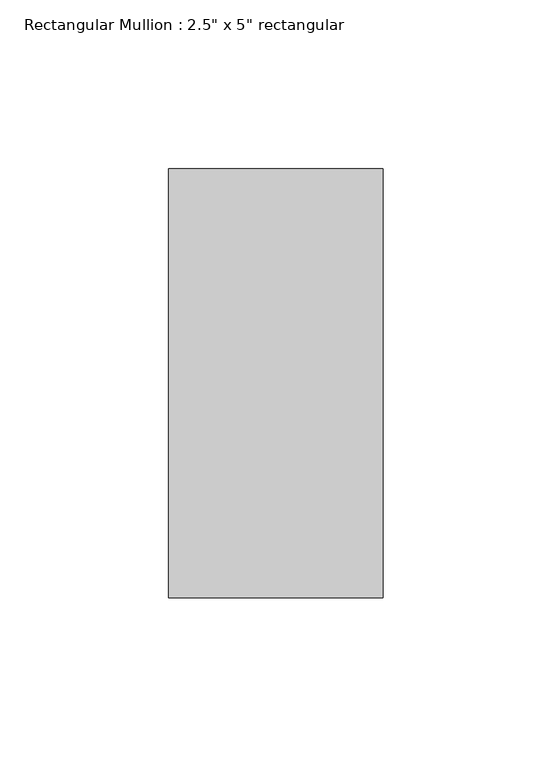
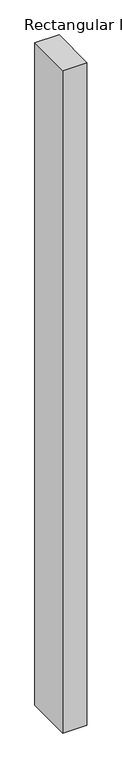
"""IFC4 building model written with IfcOpenShell, lengths in millimetres: member geometry."""

from ifc_helpers import new_model, si_unit, frame, origin, place, context, project, spatial, polyline, outline, extrude, source, transform, mapped, element, save


def member_269e6f2a(model_context):
    return source(origin(), model_context, "Body", "SweptSolid", [
        extrude(outline(polyline([(0.0, 63.5), (0.0, -63.5), (-63.5, -63.5), (-63.5, 63.5), (0.0, 63.5)])), frame((0.0, 0.0, -1843.0744962), z_axis=(0.0, 0.0, 1.0), x_axis=(1.0, 0.0, 0.0)), (0.0, 0.0, 1.0), 1843.0744962),
    ])


if __name__ == "__main__":
    model = new_model("IFC4")
    model_context = context("Model", 3, world=origin())
    ifc_project = project(units=[si_unit("LENGTHUNIT", "METRE", prefix="MILLI")], contexts=[model_context])
    site = spatial("IfcSite", under=ifc_project)
    building = spatial("IfcBuilding", under=site)
    placement = place(None, origin())
    member_shape = member_269e6f2a(model_context)
    element("IfcMember", 1, ObjectType="Rectangular Mullion : 2.5\" x 5\" rectangular", at=placement, inside=building, context=model_context, shape_type="MappedRepresentation", body=[
        mapped(member_shape, transform((0.0, 0.0, 0.0), x_axis=(1.0, 0.0, 0.0), y_axis=(0.0, 1.0, 0.0), z_axis=(0.0, 0.0, 1.0))),
    ])
    save(model, "model.ifc")

# Revit data of these elements
# Type "Rectangular Mullion : 2.5\" x 5\" rectangular"
#   built-in parameter 1007304 = 0.416667 (stored number, unit not read)
#   built-in parameter 1007301 = 0.104167 (stored number, unit not read)
#   built-in parameter 1007300 = 0.104167 (stored number, unit not read)
# Element 1 (IfcMember, "Rectangular Mullion : 2.5\" x 5\" rectangular")
#   Materials on its faces: "Aluminum"
# Materials
#   "Aluminum": class "Metal", colour RGB 247 247 247, transparency 0, Description = "Aluminum 6061", Cost = 0
